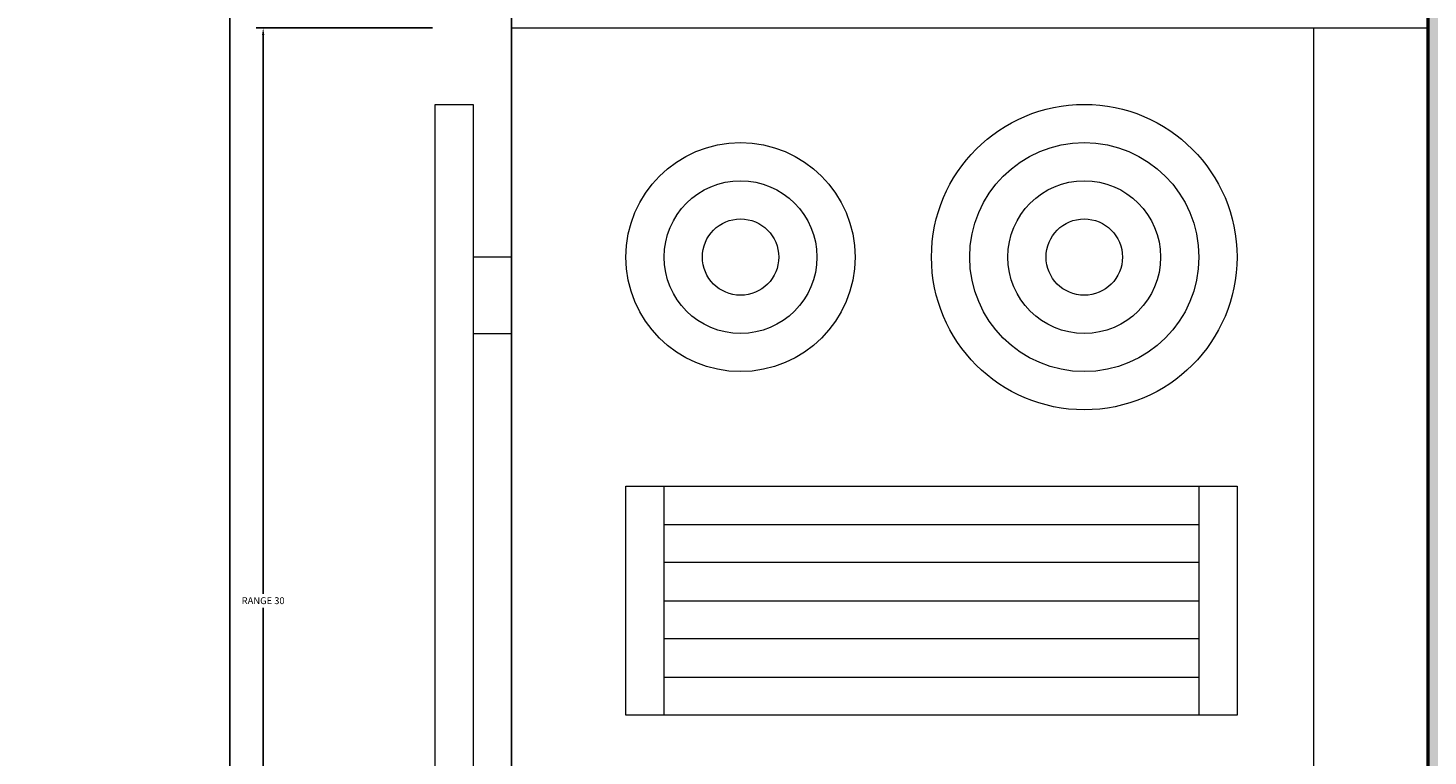
# Model space of a CAD drawing. Units: inches. Extents: x 2231 to 2461, y 2045 to 2455.
# Tile 31 of 95: x 2396 to 2433, y 2132 to 2151. Entities that reach past the tile are written whole.
import ezdxf

# ---------------------------------------------------------------- set-up
doc = ezdxf.new("R2010")
doc.units = ezdxf.units.IN
for name, color, linetype, lineweight in [('A-ANNO-DIMS', 2, 'Continuous', 18), ('A-EQPM', 8, 'Continuous', 18), ('A-FLOR-CASE', 8, 'Continuous', 25), ('A-WALL', 7, 'Continuous', 50)]:
    doc.layers.add(name, color=color, linetype=linetype, lineweight=lineweight)
doc.layers.add('A-WALL-PATT', color=18, linetype='Continuous', lineweight=13, true_color=0x000000)
doc.styles.get("Standard").update_dxf_attribs({"font": 'arial.ttf'})
doc.dimstyles.get("Standard").update_dxf_attribs({"dimtxt": 0.18, "dimasz": 0.18, "dimexe": 0.18, "dimexo": 0.0625, "dimgap": 0.09, "dimtad": 0, "dimtih": 1, "dimtoh": 1, "dimdec": 4, "dimzin": 0, "dimdsep": 46, "dimtxsty": 'Standard', "dimcen": 0.09, "dimadec": 0, "dimazin": 0, "dimtfac": 1, "dimtdec": 4, "dimtofl": 0, "dimtmove": 0, "dimatfit": 3, "dimfxl": 1, "dimtolj": 1, "dimtzin": 0, "dimarcsym": 0})

# ---------------------------------------------------------------- blocks, each defined once
blk = doc.blocks.new('Range-Oven - 30 in top')
for p, q in [((0, -3), (30, -3)), ((12, -6), (18, -6)), ((13, -20), (13, -6)), ((14, -6), (14, -20)), ((15, -20), (15, -6)), ((16, -6), (16, -20)), ((17, -20), (17, -6)), ((18, -20), (12, -20)), ((6, -24), (6, -25)), ((8, -25), (8, -24)), ((22, -25), (22, -24)), ((24, -24), (24, -25))]:
    blk.add_line(p, q)
for points in [[(0, -24), (0, 0), (30, 0), (30, -24)], [(12, -21), (12, -5), (18, -5), (18, -21)], [(2, -26), (2, -25), (28, -25), (28, -26)]]:
    blk.add_lwpolyline(points, close=True)
for centre, radius in [((6, -9), 4), ((6, -9), 3), ((24, -9), 3), ((6, -9), 2), ((24, -9), 2), ((6, -9), 1), ((24, -9), 1), ((24, -18), 4), ((6, -18), 3), ((24, -18), 3), ((6, -18), 2), ((24, -18), 2), ((6, -18), 1), ((24, -18), 1)]:
    blk.add_circle(centre, radius)
blk = doc.blocks.new('*D27')
at = {"layer": 'A-ANNO-DIMS', "color": 0, "lineweight": -2, "transparency": 16777216}
for p, q in [((2406.731, 2150.615), (2402.114, 2150.615)), ((2402.294, 2150.435), (2402.294, 2135.798)), ((2402.294, 2120.795), (2402.294, 2135.431)), ((2406.731, 2120.615), (2402.114, 2120.615))]:
    blk.add_line(p, q, dxfattribs=at)
at = {"layer": 'A-ANNO-DIMS', "color": 0, "transparency": 16777216}
for points in [[(2402.264, 2150.435), (2402.324, 2150.435), (2402.294, 2150.615)], [(2402.264, 2120.795), (2402.324, 2120.795), (2402.294, 2120.615)]]:
    blk.add_solid(points, dxfattribs=at)
at = {"layer": 'Defpoints', "color": 0, "transparency": 16777216}
for p in [(2406.794, 2150.615), (2402.294, 2120.615), (2406.794, 2120.615)]:
    blk.add_point(p, dxfattribs=at)
at = {"layer": 'A-ANNO-DIMS', "color": 0, "transparency": 16777216, "insert": (2402.294, 2135.615), "char_height": 0.18, "attachment_point": 5}
blk.add_mtext('\\A1;RANGE 30', dxfattribs=at)
blk = doc.blocks.new('*D66')
at = {"layer": 'A-ANNO-DIMS', "color": 0, "lineweight": -2, "transparency": 16777216}
for p, q in [((2348.189, 2096.895), (2348.189, 2454.645)), ((2408.794, 2096.895), (2408.794, 2454.645)), ((2348.369, 2454.465), (2378.167, 2454.465)), ((2408.614, 2454.465), (2378.815, 2454.465))]:
    blk.add_line(p, q, dxfattribs=at)
at = {"layer": 'A-ANNO-DIMS', "color": 0, "transparency": 16777216}
for points in [[(2348.369, 2454.495), (2348.369, 2454.435), (2348.189, 2454.465)], [(2408.614, 2454.495), (2408.614, 2454.435), (2408.794, 2454.465)]]:
    blk.add_solid(points, dxfattribs=at)
at = {"layer": 'Defpoints', "color": 0, "transparency": 16777216}
for p in [(2408.794, 2454.465), (2348.189, 2096.833), (2408.794, 2096.833)]:
    blk.add_point(p, dxfattribs=at)
at = {"layer": 'A-ANNO-DIMS', "color": 0, "transparency": 16777216, "insert": (2378.491, 2454.465), "char_height": 0.18, "attachment_point": 5}
blk.add_mtext('\\A1;60.6', dxfattribs=at)
blk = doc.blocks.new('*D71')
at = {"layer": 'A-ANNO-DIMS', "color": 0, "lineweight": -2, "transparency": 16777216}
for p, q in [((2401.422, 2092.979), (2401.422, 2454.645)), ((2408.794, 2096.895), (2408.794, 2454.645)), ((2401.602, 2454.465), (2404.732, 2454.465)), ((2408.614, 2454.465), (2405.483, 2454.465))]:
    blk.add_line(p, q, dxfattribs=at)
at = {"layer": 'A-ANNO-DIMS', "color": 0, "transparency": 16777216}
for points in [[(2401.602, 2454.495), (2401.602, 2454.435), (2401.422, 2454.465)], [(2408.614, 2454.495), (2408.614, 2454.435), (2408.794, 2454.465)]]:
    blk.add_solid(points, dxfattribs=at)
at = {"layer": 'Defpoints', "color": 0, "transparency": 16777216}
for p in [(2408.794, 2454.465), (2408.794, 2096.833), (2401.422, 2092.917)]:
    blk.add_point(p, dxfattribs=at)
at = {"layer": 'A-ANNO-DIMS', "color": 0, "transparency": 16777216, "insert": (2405.108, 2454.465), "char_height": 0.18, "attachment_point": 5}
blk.add_mtext('\\A1;7.371', dxfattribs=at)
blk = doc.blocks.new('*D72')
at = {"layer": 'A-ANNO-DIMS', "color": 0, "lineweight": -2, "transparency": 16777216}
for p, q in [((2384.543, 2145.12), (2384.543, 2454.645)), ((2408.794, 2150.677), (2408.794, 2454.645)), ((2384.723, 2454.465), (2396.272, 2454.465)), ((2408.614, 2454.465), (2397.064, 2454.465))]:
    blk.add_line(p, q, dxfattribs=at)
at = {"layer": 'A-ANNO-DIMS', "color": 0, "transparency": 16777216}
for points in [[(2384.723, 2454.495), (2384.723, 2454.435), (2384.543, 2454.465)], [(2408.614, 2454.495), (2408.614, 2454.435), (2408.794, 2454.465)]]:
    blk.add_solid(points, dxfattribs=at)
at = {"layer": 'Defpoints', "color": 0, "transparency": 16777216}
for p in [(2408.794, 2454.465), (2408.794, 2150.615), (2384.543, 2145.058)]:
    blk.add_point(p, dxfattribs=at)
at = {"layer": 'A-ANNO-DIMS', "color": 0, "transparency": 16777216, "insert": (2396.668, 2454.465), "char_height": 0.18, "attachment_point": 5}
blk.add_mtext('\\A1;24.25', dxfattribs=at)

msp = doc.modelspace()

# ---------------------------------------------------------------- hatches: boundary and pattern name
at = {"layer": 'A-WALL-PATT'}
h = msp.add_hatch(color=256, dxfattribs=at)
h.dxf.hatch_style = 1
h.paths.add_polyline_path([(2441.7935, 2269.1535), (2432.7935, 2269.1535), (2432.7935, 2186.8328), (2396.7935, 2186.8328), (2396.7935, 2286.8328), (2394.7935, 2286.8328), (2394.7935, 2186.8328), (2334.7935, 2186.8328), (2334.7935, 2182.8328), (2432.7935, 2182.8328), (2432.7935, 2072.8328), (2416.6639, 2072.8328), (2416.6639, 2063.8328), (2441.7935, 2063.8328)])
h.paths.add_polyline_path([(2368.6639, 2072.8328), (2367.04, 2072.8328), (2330.7942, 2072.8328), (2330.7397, 2063.8328), (2368.6639, 2063.8328)])
h.paths.add_polyline_path([(2300.7392, 2068.3328), (2300.7392, 2072.8328), (2298.7935, 2072.8328), (2294.7935, 2072.8328), (2258.7935, 2072.8328), (2258.7935, 2120.8328), (2294.7935, 2120.8328), (2298.7935, 2120.8328), (2298.7935, 2128.8328), (2294.7935, 2128.8328), (2294.7935, 2124.8328), (2258.7935, 2124.8328), (2258.7935, 2182.8328), (2294.7935, 2182.8328), (2294.7935, 2174.8328), (2298.7935, 2174.8328), (2298.7935, 2182.8328), (2304.7935, 2182.8328), (2304.7935, 2186.8328), (2258.7935, 2186.8328), (2258.7935, 2221.999), (2249.7935, 2221.999), (2249.7935, 2063.8328), (2300.7392, 2063.8328)])
h.paths.add_polyline_path([(2391.9338, 2435.8328), (2333.82, 2435.8328), (2333.82, 2426.8328), (2368.7935, 2426.8328), (2368.7935, 2374.9508), (2368.7935, 2370.8328), (2372.3935, 2370.8328), (2372.7935, 2370.8328), (2372.7935, 2426.8328), (2391.9338, 2426.8328)])
h.paths.add_polyline_path([(2441.7935, 2435.8328), (2415.9338, 2435.8328), (2415.9338, 2426.8328), (2432.7935, 2426.8328), (2432.7935, 2334.8328), (2372.7935, 2334.8328), (2372.7935, 2346.8328), (2368.7935, 2346.8328), (2368.7935, 2306.8328), (2360.7935, 2306.8328), (2360.7935, 2302.8328), (2368.7935, 2302.8328), (2372.7935, 2302.8328), (2372.7935, 2330.8328), (2432.7935, 2330.8328), (2432.7935, 2317.1535), (2441.7935, 2317.1535)])
h.paths.add_polyline_path([(2285.82, 2435.8328), (2249.7935, 2435.8328), (2249.7935, 2269.999), (2258.7935, 2269.999), (2258.7935, 2302.8328), (2318.8168, 2302.8328), (2330.7935, 2302.8328), (2330.7935, 2306.8328), (2258.7935, 2306.8328), (2258.7935, 2426.8328), (2285.82, 2426.8328)])

# ---------------------------------------------------------------- linework, layer by layer
at = {"layer": 'A-FLOR-CASE'}
msp.add_line((2408.7935, 2182.8328), (2408.7935, 2096.8328), dxfattribs=at)
at = {"layer": 'A-WALL'}
msp.add_line((2432.7935, 2182.8328), (2432.7935, 2072.8328), dxfattribs=at)

# ---------------------------------------------------------------- block references
at = {"layer": 'A-EQPM', "rotation": 270}
msp.add_blockref('Range-Oven - 30 in top', (2432.7935, 2150.6145), dxfattribs=at)

# ---------------------------------------------------------------- dimensions: what is measured, and where the dimension line sits
at = {"layer": 'A-ANNO-DIMS'}
for p1, p2, override, picture, middle in [((2348.1888, 2096.8328), (2408.7935, 2096.8328), {"dimdec": 1, "dimlfac": 1, "dimrnd": 0, "dimzin": 0, "dimdsep": 46, "dimlunit": 2}, '*D66', (2378.4912, 2454.4653)), ((2384.5428, 2145.0576), (2408.7935, 2150.6145), {"dimdec": 2, "dimlfac": 1, "dimrnd": 0, "dimzin": 0, "dimdsep": 46, "dimlunit": 2}, '*D72', (2396.6682, 2454.4653)), ((2401.4221, 2092.9167), (2408.7935, 2096.8328), {"dimdec": 3, "dimlfac": 1, "dimrnd": 0, "dimzin": 0, "dimdsep": 46, "dimlunit": 2}, '*D71', (2405.1078, 2454.4653))]:
    dim = msp.add_linear_dim(base=(2408.7935, 2454.4653), p1=p1, p2=p2, dimstyle='Standard', override=override, dxfattribs=at)
    dim.commit()
    dim.dimension.update_dxf_attribs({"geometry": picture, "text_midpoint": middle})
dim = msp.add_linear_dim(base=(2402.2935, 2120.6145), p1=(2406.7935, 2150.6145), p2=(2406.7935, 2120.6145), angle=270, text='RANGE <>', dimstyle='Standard', override={"dimdec": 0, "dimlfac": 1, "dimrnd": 0, "dimzin": 0, "dimdsep": 46, "dimlunit": 2}, dxfattribs=at)
dim.commit()
dim.dimension.update_dxf_attribs({"geometry": '*D27', "text_midpoint": (2402.2935, 2135.6145)})

doc.saveas('drawing.dxf')
